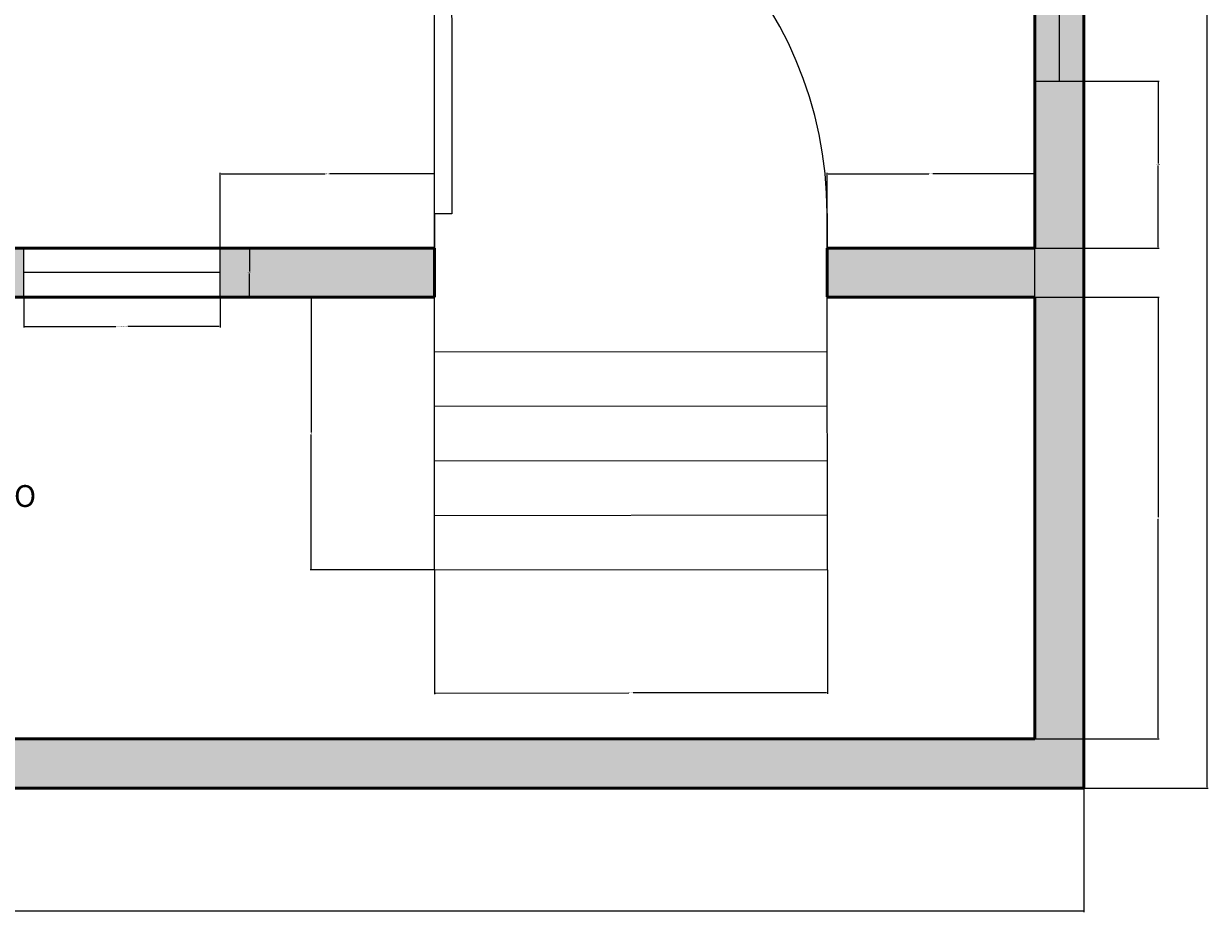
# Model space of a CAD drawing. Units: inches. Extents: x 7 to 493, y -11 to 454.
# Tile 3 of 4: x 255 to 473, y -11 to 152. Entities that reach past the tile are written whole.
import ezdxf

# ---------------------------------------------------------------- set-up
doc = ezdxf.new("R2010")
doc.units = ezdxf.units.IN
doc.header["$MEASUREMENT"] = 0
for name, color, linetype, lineweight in [('A-ANNO-DIMS', 2, 'Continuous', 18), ('A-AREA-IDEN', 7, 'Continuous', 25), ('A-FLOR-STRS', 7, 'Continuous', 25), ('A-WALL', 7, 'Continuous', 50), ('doors', 40, 'Continuous', 25), ('window', 30, 'Continuous', 18)]:
    doc.layers.add(name, color=color, linetype=linetype, lineweight=lineweight)
doc.layers.add('A-WALL-PATT', color=251, linetype='Continuous', lineweight=13, true_color=0x636466)
doc.styles.get("Standard").update_dxf_attribs({"font": 'arial.ttf'})
doc.dimstyles.get("Standard").update_dxf_attribs({"dimtxt": 0.18, "dimasz": 0.18, "dimexe": 0.18, "dimexo": 0.0625, "dimgap": 0.09, "dimtad": 0, "dimtih": 1, "dimtoh": 1, "dimdec": 4, "dimzin": 0, "dimdsep": 46, "dimtxsty": 'Standard', "dimcen": 0.09, "dimadec": 0, "dimazin": 0, "dimtfac": 1, "dimtdec": 4, "dimtofl": 0, "dimtmove": 0, "dimatfit": 3, "dimfxl": 1, "dimtolj": 1, "dimtzin": 0, "dimarcsym": 0})

# ---------------------------------------------------------------- blocks, each defined once
blk = doc.blocks.new('*U4')
for p, q in [((0, 0), (0, -6)), ((40, 0), (40, -6))]:
    blk.add_line(p, q)
blk.add_lwpolyline([(0, 0), (0, 40), (1.75, 40), (1.75, 0)], close=True)
blk.add_arc((0, 0), 40, 0, 90)
blk = doc.blocks.new('WIN-36IN')
for p, q in [((0, 0), (0, 9)), ((0, 9), (36, 9)), ((36, 9), (36, 0)), ((36, 9), (36, 4.5)), ((36, 4.5), (0, 4.5)), ((36, 0), (0, 0))]:
    blk.add_line(p, q)
blk = doc.blocks.new('*D10')
at = {"layer": 'A-ANNO-DIMS', "color": 0, "lineweight": -2, "transparency": 16777216}
for p, q in [((255.37, 101.42), (255.37, 95.91)), ((291.37, 101.42), (291.37, 95.91)), ((255.55, 96.09), (272.25, 96.09)), ((291.19, 96.09), (274.48, 96.09))]:
    blk.add_line(p, q, dxfattribs=at)
at = {"layer": 'A-ANNO-DIMS', "color": 0, "transparency": 16777216}
for points in [[(255.55, 96.12), (255.55, 96.06), (255.37, 96.09)], [(291.19, 96.12), (291.19, 96.06), (291.37, 96.09)]]:
    blk.add_solid(points, dxfattribs=at)
at = {"layer": 'Defpoints', "color": 0, "transparency": 16777216}
for p in [(255.37, 101.49), (291.37, 101.49), (291.37, 96.09)]:
    blk.add_point(p, dxfattribs=at)
at = {"layer": 'A-ANNO-DIMS', "color": 0, "transparency": 16777216, "insert": (273.37, 96.09), "char_height": 0.18, "attachment_point": 5}
blk.add_mtext('\\A1;WINDOW 36 TYP.', dxfattribs=at)
blk = doc.blocks.new('*D11')
at = {"layer": 'A-ANNO-DIMS', "color": 0, "lineweight": -2, "transparency": 16777216}
for p, q in [((291.43, 110.49), (296.95, 110.49)), ((296.77, 110.31), (296.77, 106.17)), ((296.77, 101.67), (296.77, 105.8)), ((291.43, 101.49), (296.95, 101.49))]:
    blk.add_line(p, q, dxfattribs=at)
at = {"layer": 'A-ANNO-DIMS', "color": 0, "transparency": 16777216}
for points in [[(296.74, 110.31), (296.8, 110.31), (296.77, 110.49)], [(296.74, 101.67), (296.8, 101.67), (296.77, 101.49)]]:
    blk.add_solid(points, dxfattribs=at)
at = {"layer": 'Defpoints', "color": 0, "transparency": 16777216}
for p in [(291.37, 110.49), (296.77, 110.49), (291.37, 101.49)]:
    blk.add_point(p, dxfattribs=at)
at = {"layer": 'A-ANNO-DIMS', "color": 0, "transparency": 16777216, "insert": (296.77, 105.99), "char_height": 0.18, "attachment_point": 5}
blk.add_mtext('\\A1;9 TYP.', dxfattribs=at)
blk = doc.blocks.new('*D22')
at = {"layer": 'A-ANNO-DIMS', "color": 0, "lineweight": -2, "transparency": 16777216}
for p, q in [((29.81, 11.42), (29.81, -11.29)), ((449.81, 11.42), (449.81, -11.29)), ((29.99, -11.11), (239.51, -11.11)), ((449.63, -11.11), (240.1, -11.11))]:
    blk.add_line(p, q, dxfattribs=at)
at = {"layer": 'A-ANNO-DIMS', "color": 0, "transparency": 16777216}
for points in [[(29.99, -11.08), (29.99, -11.14), (29.81, -11.11)], [(449.63, -11.08), (449.63, -11.14), (449.81, -11.11)]]:
    blk.add_solid(points, dxfattribs=at)
at = {"layer": 'Defpoints', "color": 0, "transparency": 16777216}
for p in [(29.81, 11.49), (449.81, 11.49), (449.81, -11.11)]:
    blk.add_point(p, dxfattribs=at)
at = {"layer": 'A-ANNO-DIMS', "color": 0, "transparency": 16777216, "insert": (239.81, -11.11), "char_height": 0.18, "attachment_point": 5}
blk.add_mtext('\\A1;420', dxfattribs=at)
blk = doc.blocks.new('*D23')
at = {"layer": 'A-ANNO-DIMS', "color": 0, "lineweight": -2, "transparency": 16777216}
for p, q in [((449.87, 431.49), (472.59, 431.49)), ((472.41, 431.31), (472.41, 221.67)), ((472.41, 11.67), (472.41, 221.3)), ((449.87, 11.49), (472.59, 11.49))]:
    blk.add_line(p, q, dxfattribs=at)
at = {"layer": 'A-ANNO-DIMS', "color": 0, "transparency": 16777216}
for points in [[(472.38, 431.31), (472.44, 431.31), (472.41, 431.49)], [(472.38, 11.67), (472.44, 11.67), (472.41, 11.49)]]:
    blk.add_solid(points, dxfattribs=at)
at = {"layer": 'Defpoints', "color": 0, "transparency": 16777216}
for p in [(449.81, 431.49), (472.41, 431.49), (449.81, 11.49)]:
    blk.add_point(p, dxfattribs=at)
at = {"layer": 'A-ANNO-DIMS', "color": 0, "transparency": 16777216, "insert": (472.41, 221.49), "char_height": 0.18, "attachment_point": 5}
blk.add_mtext('\\A1;420', dxfattribs=at)
blk = doc.blocks.new('*D37')
at = {"layer": 'A-ANNO-DIMS', "color": 0, "lineweight": -2, "transparency": 16777216}
for p, q in [((440.87, 101.49), (463.59, 101.49)), ((463.41, 101.31), (463.41, 61.17)), ((463.41, 20.67), (463.41, 60.8)), ((440.87, 20.49), (463.59, 20.49))]:
    blk.add_line(p, q, dxfattribs=at)
at = {"layer": 'A-ANNO-DIMS', "color": 0, "transparency": 16777216}
for points in [[(463.38, 101.31), (463.44, 101.31), (463.41, 101.49)], [(463.38, 20.67), (463.44, 20.67), (463.41, 20.49)]]:
    blk.add_solid(points, dxfattribs=at)
at = {"layer": 'Defpoints', "color": 0, "transparency": 16777216}
for p in [(440.81, 101.49), (440.81, 20.49), (463.41, 20.49)]:
    blk.add_point(p, dxfattribs=at)
at = {"layer": 'A-ANNO-DIMS', "color": 0, "transparency": 16777216, "insert": (463.41, 60.99), "char_height": 0.18, "attachment_point": 5}
blk.add_mtext('\\A1;81', dxfattribs=at)
blk = doc.blocks.new('*D38')
at = {"layer": 'A-ANNO-DIMS', "color": 0, "lineweight": -2, "transparency": 16777216}
for p, q in [((440.87, 141.11), (463.59, 141.11)), ((463.41, 140.93), (463.41, 125.98)), ((463.41, 110.67), (463.41, 125.62)), ((440.87, 110.49), (463.59, 110.49))]:
    blk.add_line(p, q, dxfattribs=at)
at = {"layer": 'A-ANNO-DIMS', "color": 0, "transparency": 16777216}
for points in [[(463.38, 140.93), (463.44, 140.93), (463.41, 141.11)], [(463.38, 110.67), (463.44, 110.67), (463.41, 110.49)]]:
    blk.add_solid(points, dxfattribs=at)
at = {"layer": 'Defpoints', "color": 0, "transparency": 16777216}
for p in [(440.81, 141.11), (440.81, 110.49), (463.41, 110.49)]:
    blk.add_point(p, dxfattribs=at)
at = {"layer": 'A-ANNO-DIMS', "color": 0, "transparency": 16777216, "insert": (463.41, 125.8), "char_height": 0.18, "attachment_point": 5}
blk.add_mtext('\\A1;30.627', dxfattribs=at)
blk = doc.blocks.new('*D46')
at = {"layer": 'A-ANNO-DIMS', "color": 0, "lineweight": -2, "transparency": 16777216}
for p, q in [((291.37, 101.55), (291.37, 124.27)), ((291.55, 124.09), (310.65, 124.09)), ((330.53, 124.09), (311.43, 124.09)), ((330.71, 101.55), (330.71, 124.27))]:
    blk.add_line(p, q, dxfattribs=at)
at = {"layer": 'A-ANNO-DIMS', "color": 0, "transparency": 16777216}
for points in [[(291.55, 124.12), (291.55, 124.06), (291.37, 124.09)], [(330.53, 124.12), (330.53, 124.06), (330.71, 124.09)]]:
    blk.add_solid(points, dxfattribs=at)
at = {"layer": 'Defpoints', "color": 0, "transparency": 16777216}
for p in [(330.71, 124.09), (291.37, 101.49), (330.71, 101.49)]:
    blk.add_point(p, dxfattribs=at)
at = {"layer": 'A-ANNO-DIMS', "color": 0, "transparency": 16777216, "insert": (311.04, 124.09), "char_height": 0.18, "attachment_point": 5}
blk.add_mtext('\\A1;39.35', dxfattribs=at)
blk = doc.blocks.new('*D47')
at = {"layer": 'A-ANNO-DIMS', "color": 0, "lineweight": -2, "transparency": 16777216}
for p, q in [((330.69, 51.42), (330.71, 28.71)), ((402.76, 51.49), (402.78, 28.77)), ((330.89, 28.89), (366.35, 28.92)), ((402.6, 28.95), (367.14, 28.92))]:
    blk.add_line(p, q, dxfattribs=at)
at = {"layer": 'A-ANNO-DIMS', "color": 0, "transparency": 16777216}
for points in [[(330.89, 28.92), (330.89, 28.86), (330.71, 28.89)], [(402.6, 28.98), (402.6, 28.92), (402.78, 28.95)]]:
    blk.add_solid(points, dxfattribs=at)
at = {"layer": 'Defpoints', "color": 0, "transparency": 16777216}
for p in [(330.69, 51.49), (402.76, 51.55), (330.71, 28.89)]:
    blk.add_point(p, dxfattribs=at)
at = {"layer": 'A-ANNO-DIMS', "color": 0, "transparency": 16777216, "insert": (366.74, 28.92), "char_height": 0.18, "attachment_point": 5}
blk.add_mtext('\\A1;72.07', dxfattribs=at)
blk = doc.blocks.new('*D48')
at = {"layer": 'A-ANNO-DIMS', "color": 0, "lineweight": -2, "transparency": 16777216}
for p, q in [((402.71, 101.55), (402.71, 124.27)), ((402.89, 124.09), (421.37, 124.09)), ((440.63, 124.09), (422.15, 124.09)), ((440.81, 101.55), (440.81, 124.27))]:
    blk.add_line(p, q, dxfattribs=at)
at = {"layer": 'A-ANNO-DIMS', "color": 0, "transparency": 16777216}
for points in [[(402.89, 124.12), (402.89, 124.06), (402.71, 124.09)], [(440.63, 124.12), (440.63, 124.06), (440.81, 124.09)]]:
    blk.add_solid(points, dxfattribs=at)
at = {"layer": 'Defpoints', "color": 0, "transparency": 16777216}
for p in [(440.81, 124.09), (402.71, 101.49), (440.81, 101.49)]:
    blk.add_point(p, dxfattribs=at)
at = {"layer": 'A-ANNO-DIMS', "color": 0, "transparency": 16777216, "insert": (421.76, 124.09), "char_height": 0.18, "attachment_point": 5}
blk.add_mtext('\\A1;38.09', dxfattribs=at)
blk = doc.blocks.new('*D49')
at = {"layer": 'A-ANNO-DIMS', "color": 0, "lineweight": -2, "transparency": 16777216}
for p, q in [((330.65, 101.49), (307.93, 101.5)), ((308.11, 101.32), (308.1, 76.68)), ((308.09, 51.68), (308.1, 76.32)), ((330.62, 51.49), (307.91, 51.5))]:
    blk.add_line(p, q, dxfattribs=at)
at = {"layer": 'A-ANNO-DIMS', "color": 0, "transparency": 16777216}
for points in [[(308.08, 101.32), (308.14, 101.32), (308.11, 101.5)], [(308.06, 51.68), (308.12, 51.68), (308.09, 51.5)]]:
    blk.add_solid(points, dxfattribs=at)
at = {"layer": 'Defpoints', "color": 0, "transparency": 16777216}
for p in [(308.11, 101.5), (330.71, 101.49), (330.69, 51.49)]:
    blk.add_point(p, dxfattribs=at)
at = {"layer": 'A-ANNO-DIMS', "color": 0, "transparency": 16777216, "insert": (308.1, 76.5), "char_height": 0.18, "attachment_point": 5}
blk.add_mtext('\\A1;50', dxfattribs=at)

msp = doc.modelspace()

# ---------------------------------------------------------------- hatches: boundary and pattern name
at = {"layer": 'A-WALL-PATT'}
h = msp.add_hatch(color=256, dxfattribs=at)
h.dxf.hatch_style = 1
h.paths.add_polyline_path([(29.8054, 11.4863), (449.8054, 11.4863), (449.8054, 431.4863), (29.8054, 431.4863)])
h.paths.add_polyline_path([(38.8054, 422.4863), (235.3054, 422.4863), (235.3054, 362.4863), (179.8054, 362.4863), (179.8054, 390.4863), (170.8054, 390.4863), (170.8054, 293.4863), (353.0513, 293.4863), (353.0513, 297.9863), (239.8054, 297.9863), (235.3054, 297.9863), (179.8054, 297.9863), (179.8054, 357.9863), (235.3054, 357.9863), (235.3054, 329.9863), (239.8054, 329.9863), (239.8054, 422.4863), (440.8054, 422.4863), (440.8054, 297.9863), (413.0513, 297.9863), (413.0513, 293.4863), (440.8054, 293.4863), (440.8054, 110.4863), (402.7135, 110.4863), (402.7135, 101.5532), (402.7135, 101.4863), (440.8054, 101.4863), (440.8054, 20.4863), (179.8054, 20.4863), (179.8054, 101.4863), (255.3658, 101.4863), (255.3658, 110.4863), (179.8054, 110.4863), (179.8054, 146.9794), (170.8054, 146.9794), (170.8054, 20.4863), (117.9037, 20.4863), (117.9037, 15.9863), (81.9037, 15.9863), (81.9037, 20.4863), (38.8054, 20.4863), (38.8054, 125.4863), (118.4942, 125.4863), (118.4942, 129.9863), (38.8054, 129.9863), (38.8054, 225.9863), (170.8054, 225.9863), (170.8054, 192.9161), (179.8054, 192.9161), (179.8054, 233.4863), (170.8054, 233.4863), (170.8054, 230.4863), (38.8054, 230.4863)], flags=16)
h.paths.add_polyline_path([(53.2938, 207.1427), (65.8095, 207.1427), (67.0594, 215.1427), (83.5282, 215.1427), (84.7782, 207.1427), (93.8095, 207.1427), (95.0594, 215.1427), (111.5282, 215.1427), (112.7782, 207.1427), (125.2938, 207.1427), (125.2938, 198.6271), (133.2938, 197.3771), (133.2938, 180.9083), (125.2938, 179.6583), (125.2938, 171.1427), (112.7782, 171.1427), (111.5282, 163.1427), (95.0594, 163.1427), (93.8095, 171.1427), (84.7782, 171.1427), (83.5282, 163.1427), (67.0594, 163.1427), (65.8095, 171.1427), (53.2938, 171.1427), (53.2938, 179.6583), (45.2938, 180.9083), (45.2938, 197.3771), (53.2938, 198.6271)], flags=0)
h.paths.add_polyline_path([(98.6154, 202.5867), (98.6833, 202.7415), (98.7209, 202.9031), (98.7311, 203.0686), (98.717, 203.2352), (98.6813, 203.3997), (98.6271, 203.5594), (98.5576, 203.7119), (98.4774, 203.8575), (98.3913, 203.9974), (98.2332, 204.2423), (98.1033, 204.4662), (98.0223, 204.7063), (98.0302, 204.9526), (98.1325, 205.1802), (98.329, 205.372), (98.3993, 205.406), (98.2782, 205.3224), (98.1805, 205.227), (98.1063, 205.1219), (98.0555, 205.0089), (98.0282, 204.8901), (98.0243, 204.7674), (98.0438, 204.6427), (98.086, 204.5175), (98.1467, 204.3914), (98.221, 204.2633), (98.3042, 204.1323), (98.4533, 203.9013), (98.6038, 203.6279), (98.7103, 203.3143), (98.7386, 202.9794), (98.6633, 202.6554)], flags=0)
h.paths.add_polyline_path([(67.2938, 216.6427), (83.2938, 216.6427), (83.45, 215.6427), (67.1375, 215.6427)], flags=0)
h.paths.add_polyline_path([(43.7938, 197.1427), (44.7938, 197.2989), (44.7938, 180.9864), (43.7938, 181.1427)], flags=0)
h.paths.add_polyline_path([(106.3833, 198.8302), (106.2808, 199.0177), (106.1587, 199.2052), (106.023, 199.3927), (105.8794, 199.5802), (105.6298, 199.9018), (105.4605, 200.1427), (105.3438, 200.33), (105.1938, 200.6147), (105.0892, 200.9776), (105.1, 201.3227), (105.1358, 201.3994), (105.0972, 201.2325), (105.0918, 201.0599), (105.1167, 200.8823), (105.169, 200.7008), (105.2456, 200.5164), (105.3438, 200.33), (105.4605, 200.1427), (105.5923, 199.9552), (105.7339, 199.7677), (105.8794, 199.5802), (106.1138, 199.2741), (106.3496, 198.9121)], flags=0)
h.paths.add_polyline_path([(124.5037, 189.2544), (124.6786, 189.213), (124.7978, 189.1834), (124.8824, 189.1635), (124.9532, 189.1515), (125.0583, 189.1432), (125.138, 189.143), (124.9529, 189.147), (124.7978, 189.1834), (124.5749, 189.2388)], flags=0)
h.paths.add_polyline_path([(95.2938, 216.6427), (111.2938, 216.6427), (111.45, 215.6427), (95.1375, 215.6427)], flags=0)
h.paths.add_polyline_path([(191.6785, 332.1221), (224.065, 332.1221), (224.065, 343.8649), (191.6785, 343.8649)], flags=8)
h.paths.add_polyline_path([(196.7522, 379.4931), (229.1387, 379.4931), (229.1387, 391.2359), (196.7522, 391.2359)], flags=8)
h.paths.add_polyline_path([(232.397, 56.3062), (260.115, 56.3062), (260.115, 68.0654), (232.397, 68.0654)], flags=8)
h.paths.add_polyline_path([(90.1783, 70.3293), (134.3492, 70.3293), (134.3492, 82.0885), (90.1783, 82.0885)], flags=8)
h.paths.add_polyline_path([(126.7274, 208.2711), (165.9297, 208.2711), (165.9297, 220.0303), (126.7274, 220.0303)], flags=8)
h.paths.add_polyline_path([(261.4741, 205.6105), (297.4786, 205.6105), (297.4786, 217.3697), (261.4741, 217.3697)], flags=8)
h.paths.add_polyline_path([(77.3838, 283.1969), (106.5561, 283.1969), (106.5561, 294.9561), (77.3838, 294.9561)], flags=8)
h.paths.add_polyline_path([(357.5163, 353.5423), (386.6886, 353.5423), (386.6886, 365.3015), (357.5163, 365.3015)], flags=8)
h = msp.add_hatch(color=256, dxfattribs=at)
h.dxf.hatch_style = 1
h.paths.add_polyline_path([(330.7135, 110.4863), (291.3658, 110.4863), (291.3658, 105.9863), (291.3658, 101.4863), (330.7135, 101.4863)])

# ---------------------------------------------------------------- linework, layer by layer
at = {"layer": 'A-FLOR-STRS'}
for p, q in [((330.6856, 51.4863), (330.7321, 101.5532)), ((402.7599, 51.5532), (402.7135, 101.5532)), ((330.7228, 91.4863), (402.7227, 91.5532)), ((330.7134, 81.4863), (402.732, 81.5532)), ((330.7041, 71.4863), (402.7413, 71.5532)), ((330.6949, 61.4863), (402.7506, 61.5532)), ((330.6856, 51.4863), (402.7599, 51.5532))]:
    msp.add_line(p, q, dxfattribs=at)
at = {"layer": 'A-WALL'}
for p, q in [((440.8054, 293.4863), (440.8054, 110.4863)), ((179.8054, 110.4863), (330.7135, 110.4863)), ((330.7135, 110.4863), (330.7135, 101.4863)), ((402.7135, 110.4863), (440.8054, 110.4863)), ((402.7135, 101.5532), (402.7135, 110.4863)), ((179.8054, 101.4863), (330.7135, 101.4863)), ((402.7135, 101.4863), (440.8054, 101.4863)), ((440.8054, 101.4863), (440.8054, 20.4863)), ((440.8054, 20.4863), (179.8054, 20.4863))]:
    msp.add_line(p, q, dxfattribs=at)
msp.add_lwpolyline([(29.8054, 431.4863), (449.8054, 431.4863), (449.8054, 11.4863), (29.8054, 11.4863)], close=True, dxfattribs=at)

# ---------------------------------------------------------------- block references
at = {"layer": 'doors', "xscale": 1.799999418286923, "yscale": 1.799999418286923, "zscale": 1.799999418286923, "rotation": 0.026594711782106}
msp.add_blockref('*U4', (330.7085, 116.7863), dxfattribs=at)
at = {"layer": 'window', "extrusion": (0, 0, -1), "zscale": -1, "rotation": 269.9999999999964}
msp.add_blockref('WIN-36IN', (-449.8057, 177.1129), dxfattribs=at)
at = {"layer": 'window'}
msp.add_blockref('WIN-36IN', (255.366, 101.486), dxfattribs=at)

# ---------------------------------------------------------------- texts
at = {"layer": 'A-AREA-IDEN', "insert": (233.0554, 67.0277), "char_height": 0.2, "attachment_point": 1}
msp.add_mtext_dynamic_manual_height_columns("{\\H20x; PORTICO\\P16' X10'}", width=58.591086, gutter_width=1, heights=[0], dxfattribs=at)

# ---------------------------------------------------------------- dimensions: what is measured, and where the dimension line sits
at = {"layer": 'A-ANNO-DIMS'}
for base, p1, p2, angle, override, picture, middle in [((472.4054, 431.4863), (449.8054, 11.4863), (449.8054, 431.4863), 90, {"dimdec": 0, "dimlfac": 1, "dimrnd": 0, "dimzin": 0, "dimdsep": 46, "dimlunit": 2}, '*D23', (472.4054, 221.4863)), ((463.4054, 110.4863), (440.8054, 141.1131), (440.8054, 110.4863), 270, {"dimdec": 3, "dimlfac": 1, "dimrnd": 0, "dimzin": 0, "dimdsep": 46, "dimlunit": 2}, '*D38', (463.4054, 125.7997)), ((330.7135, 124.0863), (291.3658, 101.4863), (330.7135, 101.4863), 0, {"dimdec": 2, "dimlfac": 1, "dimrnd": 0, "dimzin": 0, "dimdsep": 46, "dimlunit": 2}, '*D46', (311.0396, 124.0863)), ((308.1135, 101.4989), (330.6856, 51.4863), (330.7135, 101.4863), 89.968015, {"dimdec": 0, "dimlfac": 1, "dimrnd": 0, "dimzin": 0, "dimdsep": 46, "dimlunit": 2}, '*D49', (308.0995, 76.4989)), ((463.4054, 20.4863), (440.8054, 101.4863), (440.8054, 20.4863), 270, {"dimdec": 0, "dimlfac": 1, "dimrnd": 0, "dimzin": 0, "dimdsep": 46, "dimlunit": 2}, '*D37', (463.4054, 60.9863)), ((330.7066, 28.8863), (402.7599, 51.5532), (330.6856, 51.4863), 180.053189, {"dimdec": 2, "dimlfac": 1, "dimrnd": 0, "dimzin": 0, "dimdsep": 46, "dimlunit": 2}, '*D47', (366.7437, 28.9197))]:
    dim = msp.add_linear_dim(base=base, p1=p1, p2=p2, angle=angle, dimstyle='Standard', override=override, dxfattribs=at)
    dim.commit()
    dim.dimension.update_dxf_attribs({"geometry": picture, "text_midpoint": middle})
for base, p1, p2, override, picture, middle in [((440.8054, 124.0863), (402.7135, 101.4863), (440.8054, 101.4863), {"dimdec": 2, "dimlfac": 1, "dimrnd": 0, "dimzin": 0, "dimdsep": 46, "dimlunit": 2}, '*D48', (421.7594, 124.0863)), ((449.8054, -11.1137), (29.8054, 11.4863), (449.8054, 11.4863), {"dimdec": 0, "dimlfac": 1, "dimrnd": 0, "dimzin": 0, "dimdsep": 46, "dimlunit": 2}, '*D22', (239.8054, -11.1137))]:
    dim = msp.add_linear_dim(base=base, p1=p1, p2=p2, dimstyle='Standard', override=override, dxfattribs=at)
    dim.commit()
    dim.dimension.update_dxf_attribs({"geometry": picture, "text_midpoint": middle})
dim = msp.add_linear_dim(base=(296.7658, 110.4863), p1=(291.3658, 101.4863), p2=(291.3658, 110.4863), angle=90, text='<> TYP.', dimstyle='Standard', override={"dimdec": 0, "dimlfac": 1, "dimrnd": 0, "dimzin": 0, "dimdsep": 46, "dimlunit": 2}, dxfattribs=at)
dim.commit()
dim.dimension.update_dxf_attribs({"geometry": '*D11', "text_midpoint": (296.7658, 105.9863)})
dim = msp.add_linear_dim(base=(291.3658, 96.0863), p1=(255.3658, 101.4863), p2=(291.3658, 101.4863), text='WINDOW <> TYP.', dimstyle='Standard', override={"dimdec": 0, "dimlfac": 1, "dimrnd": 0, "dimzin": 0, "dimdsep": 46, "dimlunit": 2}, dxfattribs=at)
dim.commit()
dim.dimension.update_dxf_attribs({"geometry": '*D10', "text_midpoint": (273.3658, 96.0863)})

doc.saveas('drawing.dxf')
